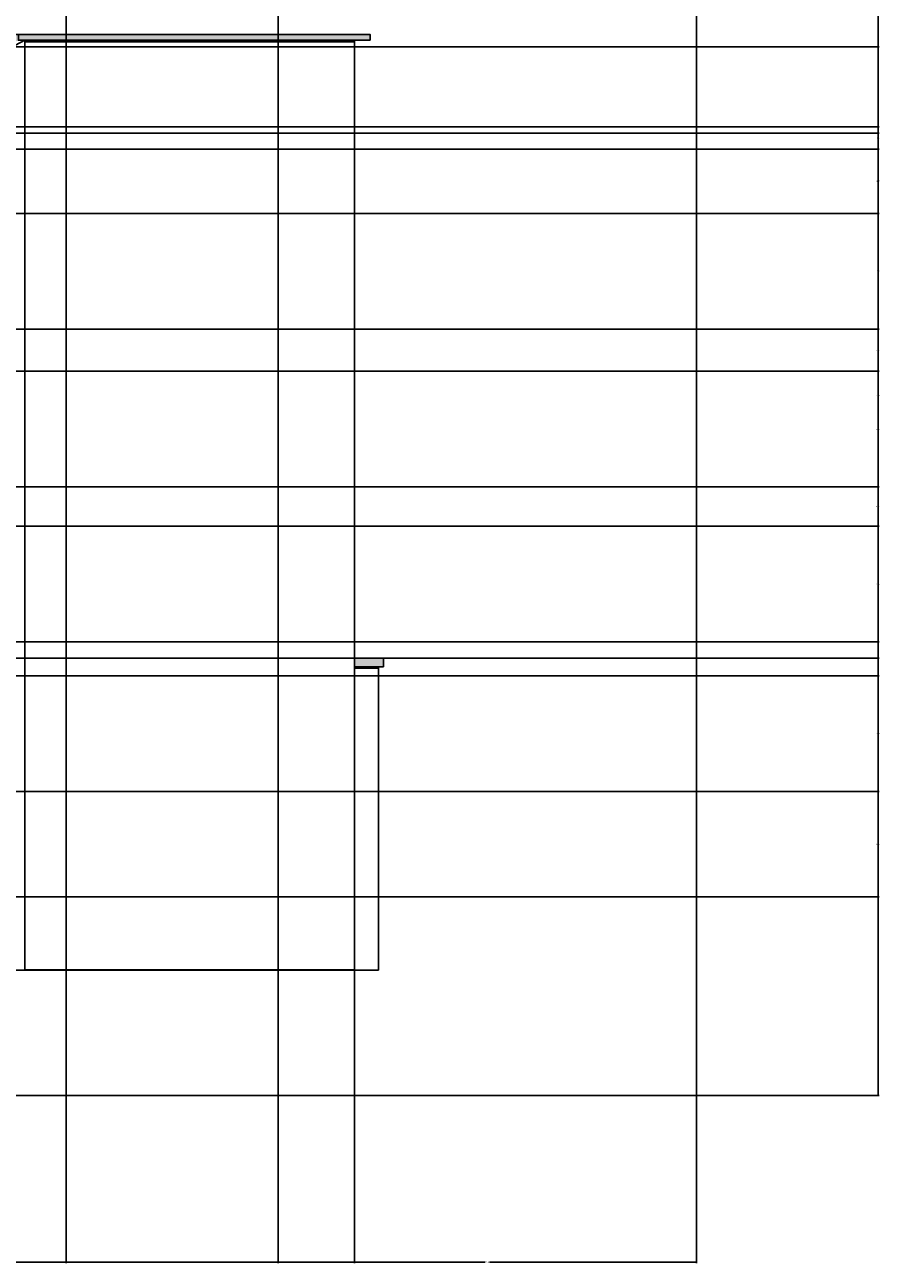
# Model space of a CAD drawing. Units: millimetres. Extents: x 171 to 1599, y 973 to 1509.
# Tile 6 of 7: x 1445 to 1599, y 973 to 1196. Entities that reach past the tile are written whole.
import ezdxf

# ---------------------------------------------------------------- set-up
doc = ezdxf.new("R2010")
doc.units = ezdxf.units.MM
for name, color, linetype, lineweight in [('A-ANNO-DIMS', 2, 'Continuous', 18), ('A-ELEV', 7, 'Continuous', 25), ('A-ELEV-FILL', 252, 'Continuous', 13)]:
    doc.layers.add(name, color=color, linetype=linetype, lineweight=lineweight)
doc.styles.get("Standard").update_dxf_attribs({"font": 'arial.ttf'})
doc.dimstyles.get("Standard").update_dxf_attribs({"dimtxt": 0.18, "dimasz": 0.18, "dimexe": 0.18, "dimexo": 0.0625, "dimgap": 0.09, "dimtad": 0, "dimtih": 1, "dimtoh": 1, "dimdec": 1, "dimzin": 0, "dimdsep": 46, "dimlunit": 3, "dimtxsty": 'Standard', "dimcen": 0.09, "dimadec": 0, "dimazin": 0, "dimtfac": 1, "dimtdec": 1, "dimtofl": 0, "dimtmove": 0, "dimatfit": 3, "dimfxl": 1, "dimtolj": 1, "dimtzin": 0, "dimarcsym": 0})

# ---------------------------------------------------------------- blocks, each defined once
blk = doc.blocks.new('*D1')
at = {"layer": 'A-ANNO-DIMS', "color": 0, "lineweight": -2, "transparency": 16777216}
for p, q in [((980.93, 1194.55), (980.93, 1508.31)), ((981.11, 1508.13), (1274.61, 1508.13)), ((1568.85, 1508.13), (1275.36, 1508.13)), ((1569.03, 1215.31), (1569.03, 1508.31))]:
    blk.add_line(p, q, dxfattribs=at)
at = {"layer": 'A-ANNO-DIMS', "color": 0, "transparency": 16777216}
for points in [[(981.11, 1508.16), (981.11, 1508.1), (980.93, 1508.13)], [(1568.85, 1508.16), (1568.85, 1508.1), (1569.03, 1508.13)]]:
    blk.add_solid(points, dxfattribs=at)
at = {"layer": 'Defpoints', "color": 0, "transparency": 16777216}
for p in [(1569.03, 1508.13), (1569.03, 1215.25), (980.93, 1194.49)]:
    blk.add_point(p, dxfattribs=at)
at = {"layer": 'A-ANNO-DIMS', "color": 0, "transparency": 16777216, "insert": (1274.98, 1508.13), "char_height": 0.18, "attachment_point": 5}
blk.add_mtext('\\A1;588.1', dxfattribs=at)
blk = doc.blocks.new('*D2')
at = {"layer": 'A-ANNO-DIMS', "color": 0, "lineweight": -2, "transparency": 16777216}
for p, q in [((1043.70287, 1478.130098), (1599.212656, 1478.130098)), ((1599.032656, 1477.950098), (1599.032656, 1240.959874)), ((1599.032656, 1003.60965), (1599.032656, 1240.599874)), ((1348.449149, 1003.42965), (1599.212656, 1003.42965))]:
    blk.add_line(p, q, dxfattribs=at)
at = {"layer": 'A-ANNO-DIMS', "color": 0, "transparency": 16777216}
for points in [[(1599.002656, 1477.950098), (1599.062656, 1477.950098), (1599.032656, 1478.130098)], [(1599.002656, 1003.60965), (1599.062656, 1003.60965), (1599.032656, 1003.42965)]]:
    blk.add_solid(points, dxfattribs=at)
at = {"layer": 'Defpoints', "color": 0, "transparency": 16777216}
for p in [(1043.64037, 1478.130098), (1599.032656, 1478.130098), (1348.386649, 1003.42965)]:
    blk.add_point(p, dxfattribs=at)
at = {"layer": 'A-ANNO-DIMS', "color": 0, "transparency": 16777216, "insert": (1599.032656, 1240.779874), "char_height": 0.18, "attachment_point": 5}
blk.add_mtext('\\A1;474.7', dxfattribs=at)
blk = doc.blocks.new('*D10')
at = {"layer": 'A-ANNO-DIMS', "color": 0, "lineweight": -2, "transparency": 16777216}
for p, q in [((1441.28, 1082.17), (1441.28, 973.25)), ((1504.77, 1026.01), (1504.77, 973.25)), ((1441.46, 973.43), (1472.63, 973.43)), ((1504.59, 973.43), (1473.42, 973.43))]:
    blk.add_line(p, q, dxfattribs=at)
at = {"layer": 'A-ANNO-DIMS', "color": 0, "transparency": 16777216}
for points in [[(1441.46, 973.46), (1441.46, 973.4), (1441.28, 973.43)], [(1504.59, 973.46), (1504.59, 973.4), (1504.77, 973.43)]]:
    blk.add_solid(points, dxfattribs=at)
at = {"layer": 'Defpoints', "color": 0, "transparency": 16777216}
for p in [(1441.28, 1082.23), (1504.77, 1026.08), (1504.77, 973.43)]:
    blk.add_point(p, dxfattribs=at)
at = {"layer": 'A-ANNO-DIMS', "color": 0, "transparency": 16777216, "insert": (1473.02, 973.43), "char_height": 0.18, "attachment_point": 5}
blk.add_mtext('\\A1;63.49', dxfattribs=at)
blk = doc.blocks.new('*D58')
at = {"layer": 'A-ANNO-DIMS', "color": 0, "lineweight": -2, "transparency": 16777216}
for p, q in [((1452.86, 1194.43), (1452.86, 973.25)), ((1416.22, 1192.2), (1416.22, 973.25)), ((1416.4, 973.43), (1434.08, 973.43)), ((1452.68, 973.43), (1435, 973.43))]:
    blk.add_line(p, q, dxfattribs=at)
at = {"layer": 'A-ANNO-DIMS', "color": 0, "transparency": 16777216}
for points in [[(1416.4, 973.46), (1416.4, 973.4), (1416.22, 973.43)], [(1452.68, 973.46), (1452.68, 973.4), (1452.86, 973.43)]]:
    blk.add_solid(points, dxfattribs=at)
at = {"layer": 'Defpoints', "color": 0, "transparency": 16777216}
for p in [(1452.86, 1194.49), (1416.22, 1192.27), (1452.86, 973.43)]:
    blk.add_point(p, dxfattribs=at)
at = {"layer": 'A-ANNO-DIMS', "color": 0, "transparency": 16777216, "insert": (1434.54, 973.43), "char_height": 0.18, "attachment_point": 5}
blk.add_mtext('\\A1;36.636', dxfattribs=at)
blk = doc.blocks.new('*D59')
at = {"layer": 'A-ANNO-DIMS', "color": 0, "lineweight": -2, "transparency": 16777216}
for p, q in [((1452.86, 1194.43), (1452.86, 973.25)), ((1491.01, 1194.43), (1491.01, 973.25)), ((1453.04, 973.43), (1471.47, 973.43)), ((1490.83, 973.43), (1472.4, 973.43))]:
    blk.add_line(p, q, dxfattribs=at)
at = {"layer": 'A-ANNO-DIMS', "color": 0, "transparency": 16777216}
for points in [[(1453.04, 973.46), (1453.04, 973.4), (1452.86, 973.43)], [(1490.83, 973.46), (1490.83, 973.4), (1491.01, 973.43)]]:
    blk.add_solid(points, dxfattribs=at)
at = {"layer": 'Defpoints', "color": 0, "transparency": 16777216}
for p in [(1452.86, 1194.49), (1491.01, 1194.49), (1491.01, 973.43)]:
    blk.add_point(p, dxfattribs=at)
at = {"layer": 'A-ANNO-DIMS', "color": 0, "transparency": 16777216, "insert": (1471.94, 973.43), "char_height": 0.18, "attachment_point": 5}
blk.add_mtext('\\A1;38.156', dxfattribs=at)
blk = doc.blocks.new('*D60')
at = {"layer": 'A-ANNO-DIMS', "color": 0, "lineweight": -2, "transparency": 16777216}
for p, q in [((1566.36, 1203.74), (1566.36, 973.25)), ((1491.01, 1194.43), (1491.01, 973.25)), ((1491.19, 973.43), (1528.29, 973.43)), ((1566.18, 973.43), (1529.08, 973.43))]:
    blk.add_line(p, q, dxfattribs=at)
at = {"layer": 'A-ANNO-DIMS', "color": 0, "transparency": 16777216}
for points in [[(1491.19, 973.46), (1491.19, 973.4), (1491.01, 973.43)], [(1566.18, 973.46), (1566.18, 973.4), (1566.36, 973.43)]]:
    blk.add_solid(points, dxfattribs=at)
at = {"layer": 'Defpoints', "color": 0, "transparency": 16777216}
for p in [(1566.36, 1203.8), (1491.01, 1194.49), (1566.36, 973.43)]:
    blk.add_point(p, dxfattribs=at)
at = {"layer": 'A-ANNO-DIMS', "color": 0, "transparency": 16777216, "insert": (1528.69, 973.43), "char_height": 0.18, "attachment_point": 5}
blk.add_mtext('\\A1;75.35', dxfattribs=at)
blk = doc.blocks.new('*D62')
at = {"layer": 'A-ANNO-DIMS', "color": 0, "lineweight": -2, "transparency": 16777216}
for p, q in [((1416.28, 1290.48), (1599.21, 1290.48)), ((1599.03, 1290.3), (1599.03, 1241.56)), ((1599.03, 1192.45), (1599.03, 1241.19)), ((1416.28, 1192.27), (1599.21, 1192.27))]:
    blk.add_line(p, q, dxfattribs=at)
at = {"layer": 'A-ANNO-DIMS', "color": 0, "transparency": 16777216}
for points in [[(1599, 1290.3), (1599.06, 1290.3), (1599.03, 1290.48)], [(1599, 1192.45), (1599.06, 1192.45), (1599.03, 1192.27)]]:
    blk.add_solid(points, dxfattribs=at)
at = {"layer": 'Defpoints', "color": 0, "transparency": 16777216}
for p in [(1416.22, 1290.48), (1599.03, 1290.48), (1416.22, 1192.27)]:
    blk.add_point(p, dxfattribs=at)
at = {"layer": 'A-ANNO-DIMS', "color": 0, "transparency": 16777216, "insert": (1599.03, 1241.38), "char_height": 0.18, "attachment_point": 5}
blk.add_mtext('\\A1;98.22', dxfattribs=at)
blk = doc.blocks.new('*D86')
at = {"layer": 'A-ANNO-DIMS', "color": 0, "lineweight": -2, "transparency": 16777216}
for p, q in [((1441.34, 1176.74), (1599.21, 1176.74)), ((1599.03, 1176.56), (1599.03, 1129.67)), ((1599.03, 1082.41), (1599.03, 1129.31)), ((1441.34, 1082.23), (1599.21, 1082.23))]:
    blk.add_line(p, q, dxfattribs=at)
at = {"layer": 'A-ANNO-DIMS', "color": 0, "transparency": 16777216}
for points in [[(1599, 1176.56), (1599.06, 1176.56), (1599.03, 1176.74)], [(1599, 1082.41), (1599.06, 1082.41), (1599.03, 1082.23)]]:
    blk.add_solid(points, dxfattribs=at)
at = {"layer": 'Defpoints', "color": 0, "transparency": 16777216}
for p in [(1441.28, 1176.74), (1599.03, 1176.74), (1441.28, 1082.23)]:
    blk.add_point(p, dxfattribs=at)
at = {"layer": 'A-ANNO-DIMS', "color": 0, "transparency": 16777216, "insert": (1599.03, 1129.49), "char_height": 0.18, "attachment_point": 5}
blk.add_mtext('\\A1;94.51', dxfattribs=at)
blk = doc.blocks.new('*D87')
at = {"layer": 'A-ANNO-DIMS', "color": 0, "lineweight": -2, "transparency": 16777216}
for p, q in [((1281.3, 1058.21), (1599.21, 1058.21)), ((1599.03, 1058.03), (1599.03, 1048.91)), ((1599.03, 1039.43), (1599.03, 1048.55)), ((1294.3, 1039.25), (1599.21, 1039.25))]:
    blk.add_line(p, q, dxfattribs=at)
at = {"layer": 'A-ANNO-DIMS', "color": 0, "transparency": 16777216}
for points in [[(1599, 1058.03), (1599.06, 1058.03), (1599.03, 1058.21)], [(1599, 1039.43), (1599.06, 1039.43), (1599.03, 1039.25)]]:
    blk.add_solid(points, dxfattribs=at)
at = {"layer": 'Defpoints', "color": 0, "transparency": 16777216}
for p in [(1281.24, 1058.21), (1599.03, 1058.21), (1294.24, 1039.25)]:
    blk.add_point(p, dxfattribs=at)
at = {"layer": 'A-ANNO-DIMS', "color": 0, "transparency": 16777216, "insert": (1599.03, 1048.73), "char_height": 0.18, "attachment_point": 5}
blk.add_mtext('\\A1;18.956', dxfattribs=at)
blk = doc.blocks.new('*D88')
at = {"layer": 'A-ANNO-DIMS', "color": 0, "lineweight": -2, "transparency": 16777216}
for p, q in [((1281.3, 1079.04), (1599.21, 1079.04)), ((1599.03, 1078.86), (1599.03, 1068.8)), ((1599.03, 1058.39), (1599.03, 1068.44)), ((1281.3, 1058.21), (1599.21, 1058.21))]:
    blk.add_line(p, q, dxfattribs=at)
at = {"layer": 'A-ANNO-DIMS', "color": 0, "transparency": 16777216}
for points in [[(1599, 1078.86), (1599.06, 1078.86), (1599.03, 1079.04)], [(1599, 1058.39), (1599.06, 1058.39), (1599.03, 1058.21)]]:
    blk.add_solid(points, dxfattribs=at)
at = {"layer": 'Defpoints', "color": 0, "transparency": 16777216}
for p in [(1281.24, 1079.04), (1599.03, 1079.04), (1281.24, 1058.21)]:
    blk.add_point(p, dxfattribs=at)
at = {"layer": 'A-ANNO-DIMS', "color": 0, "transparency": 16777216, "insert": (1599.03, 1068.62), "char_height": 0.18, "attachment_point": 5}
blk.add_mtext('\\A1;20.833', dxfattribs=at)
blk = doc.blocks.new('*D89')
at = {"layer": 'A-ANNO-DIMS', "color": 0, "lineweight": -2, "transparency": 16777216}
for p, q in [((1281.3, 1085.12), (1599.21, 1085.12)), ((1599.03, 1084.94), (1599.03, 1082.26)), ((1599.03, 1079.22), (1599.03, 1081.9)), ((1281.3, 1079.04), (1599.21, 1079.04))]:
    blk.add_line(p, q, dxfattribs=at)
at = {"layer": 'A-ANNO-DIMS', "color": 0, "transparency": 16777216}
for points in [[(1599, 1084.94), (1599.06, 1084.94), (1599.03, 1085.12)], [(1599, 1079.22), (1599.06, 1079.22), (1599.03, 1079.04)]]:
    blk.add_solid(points, dxfattribs=at)
at = {"layer": 'Defpoints', "color": 0, "transparency": 16777216}
for p in [(1281.24, 1085.12), (1599.03, 1085.12), (1281.24, 1079.04)]:
    blk.add_point(p, dxfattribs=at)
at = {"layer": 'A-ANNO-DIMS', "color": 0, "transparency": 16777216, "insert": (1599.03, 1082.08), "char_height": 0.18, "attachment_point": 5}
blk.add_mtext('\\A1;6.079', dxfattribs=at)
blk = doc.blocks.new('*D90')
at = {"layer": 'A-ANNO-DIMS', "color": 0, "lineweight": -2, "transparency": 16777216}
for p, q in [((1281.3, 1105.95), (1599.21, 1105.95)), ((1599.03, 1105.77), (1599.03, 1095.72)), ((1599.03, 1085.3), (1599.03, 1095.35)), ((1281.3, 1085.12), (1599.21, 1085.12))]:
    blk.add_line(p, q, dxfattribs=at)
at = {"layer": 'A-ANNO-DIMS', "color": 0, "transparency": 16777216}
for points in [[(1599, 1105.77), (1599.06, 1105.77), (1599.03, 1105.95)], [(1599, 1085.3), (1599.06, 1085.3), (1599.03, 1085.12)]]:
    blk.add_solid(points, dxfattribs=at)
at = {"layer": 'Defpoints', "color": 0, "transparency": 16777216}
for p in [(1281.24, 1105.95), (1599.03, 1105.95), (1281.24, 1085.12)]:
    blk.add_point(p, dxfattribs=at)
at = {"layer": 'A-ANNO-DIMS', "color": 0, "transparency": 16777216, "insert": (1599.03, 1095.53), "char_height": 0.18, "attachment_point": 5}
blk.add_mtext('\\A1;20.833', dxfattribs=at)
blk = doc.blocks.new('*D91')
at = {"layer": 'A-ANNO-DIMS', "color": 0, "lineweight": -2, "transparency": 16777216}
for p, q in [((1281.3, 1113.05), (1599.21, 1113.05)), ((1599.03, 1112.87), (1599.03, 1109.68)), ((1599.03, 1106.13), (1599.03, 1109.32)), ((1281.3, 1105.95), (1599.21, 1105.95))]:
    blk.add_line(p, q, dxfattribs=at)
at = {"layer": 'A-ANNO-DIMS', "color": 0, "transparency": 16777216}
for points in [[(1599, 1112.87), (1599.06, 1112.87), (1599.03, 1113.05)], [(1599, 1106.13), (1599.06, 1106.13), (1599.03, 1105.95)]]:
    blk.add_solid(points, dxfattribs=at)
at = {"layer": 'Defpoints', "color": 0, "transparency": 16777216}
for p in [(1281.24, 1113.05), (1599.03, 1113.05), (1281.24, 1105.95)]:
    blk.add_point(p, dxfattribs=at)
at = {"layer": 'A-ANNO-DIMS', "color": 0, "transparency": 16777216, "insert": (1599.03, 1109.5), "char_height": 0.18, "attachment_point": 5}
blk.add_mtext('\\A1;7.102', dxfattribs=at)
blk = doc.blocks.new('*D92')
at = {"layer": 'A-ANNO-DIMS', "color": 0, "lineweight": -2, "transparency": 16777216}
for p, q in [((1281.3, 1133.89), (1599.21, 1133.89)), ((1599.03, 1133.71), (1599.03, 1123.65)), ((1599.03, 1113.23), (1599.03, 1123.29)), ((1281.3, 1113.05), (1599.21, 1113.05))]:
    blk.add_line(p, q, dxfattribs=at)
at = {"layer": 'A-ANNO-DIMS', "color": 0, "transparency": 16777216}
for points in [[(1599, 1133.71), (1599.06, 1133.71), (1599.03, 1133.89)], [(1599, 1113.23), (1599.06, 1113.23), (1599.03, 1113.05)]]:
    blk.add_solid(points, dxfattribs=at)
at = {"layer": 'Defpoints', "color": 0, "transparency": 16777216}
for p in [(1281.24, 1133.89), (1599.03, 1133.89), (1281.24, 1113.05)]:
    blk.add_point(p, dxfattribs=at)
at = {"layer": 'A-ANNO-DIMS', "color": 0, "transparency": 16777216, "insert": (1599.03, 1123.47), "char_height": 0.18, "attachment_point": 5}
blk.add_mtext('\\A1;20.833', dxfattribs=at)
blk = doc.blocks.new('*D93')
at = {"layer": 'A-ANNO-DIMS', "color": 0, "lineweight": -2, "transparency": 16777216}
for p, q in [((1281.3, 1141.45), (1599.21, 1141.45)), ((1599.03, 1141.27), (1599.03, 1137.85)), ((1599.03, 1134.07), (1599.03, 1137.49)), ((1281.3, 1133.89), (1599.21, 1133.89))]:
    blk.add_line(p, q, dxfattribs=at)
at = {"layer": 'A-ANNO-DIMS', "color": 0, "transparency": 16777216}
for points in [[(1599, 1141.27), (1599.06, 1141.27), (1599.03, 1141.45)], [(1599, 1134.07), (1599.06, 1134.07), (1599.03, 1133.89)]]:
    blk.add_solid(points, dxfattribs=at)
at = {"layer": 'Defpoints', "color": 0, "transparency": 16777216}
for p in [(1281.24, 1141.45), (1599.03, 1141.45), (1281.24, 1133.89)]:
    blk.add_point(p, dxfattribs=at)
at = {"layer": 'A-ANNO-DIMS', "color": 0, "transparency": 16777216, "insert": (1599.03, 1137.67), "char_height": 0.18, "attachment_point": 5}
blk.add_mtext('\\A1;7.567', dxfattribs=at)
blk = doc.blocks.new('*D94')
at = {"layer": 'A-ANNO-DIMS', "color": 0, "lineweight": -2, "transparency": 16777216}
for p, q in [((1281.3, 1162.29), (1599.21, 1162.29)), ((1599.03, 1162.11), (1599.03, 1152.05)), ((1599.03, 1141.63), (1599.03, 1151.69)), ((1281.3, 1141.45), (1599.21, 1141.45))]:
    blk.add_line(p, q, dxfattribs=at)
at = {"layer": 'A-ANNO-DIMS', "color": 0, "transparency": 16777216}
for points in [[(1599, 1162.11), (1599.06, 1162.11), (1599.03, 1162.29)], [(1599, 1141.63), (1599.06, 1141.63), (1599.03, 1141.45)]]:
    blk.add_solid(points, dxfattribs=at)
at = {"layer": 'Defpoints', "color": 0, "transparency": 16777216}
for p in [(1281.24, 1162.29), (1599.03, 1162.29), (1281.24, 1141.45)]:
    blk.add_point(p, dxfattribs=at)
at = {"layer": 'A-ANNO-DIMS', "color": 0, "transparency": 16777216, "insert": (1599.03, 1151.87), "char_height": 0.18, "attachment_point": 5}
blk.add_mtext('\\A1;20.833', dxfattribs=at)
blk = doc.blocks.new('*D95')
at = {"layer": 'A-ANNO-DIMS', "color": 0, "lineweight": -2, "transparency": 16777216}
for p, q in [((1294.3, 1173.87), (1599.21, 1173.87)), ((1599.03, 1173.69), (1599.03, 1168.26)), ((1599.03, 1162.47), (1599.03, 1167.9)), ((1281.3, 1162.29), (1599.21, 1162.29))]:
    blk.add_line(p, q, dxfattribs=at)
at = {"layer": 'A-ANNO-DIMS', "color": 0, "transparency": 16777216}
for points in [[(1599, 1173.69), (1599.06, 1173.69), (1599.03, 1173.87)], [(1599, 1162.47), (1599.06, 1162.47), (1599.03, 1162.29)]]:
    blk.add_solid(points, dxfattribs=at)
at = {"layer": 'Defpoints', "color": 0, "transparency": 16777216}
for p in [(1294.24, 1173.87), (1599.03, 1173.87), (1281.24, 1162.29)]:
    blk.add_point(p, dxfattribs=at)
at = {"layer": 'A-ANNO-DIMS', "color": 0, "transparency": 16777216, "insert": (1599.03, 1168.08), "char_height": 0.18, "attachment_point": 5}
blk.add_mtext('\\A1;11.587', dxfattribs=at)
blk = doc.blocks.new('*D96')
at = {"layer": 'A-ANNO-DIMS', "color": 0, "lineweight": -2, "transparency": 16777216}
for p, q in [((1298.3, 1177.87), (1599.21, 1177.87)), ((1599.03, 1177.69), (1599.03, 1176.05)), ((1599.03, 1174.05), (1599.03, 1175.69)), ((1294.3, 1173.87), (1599.21, 1173.87))]:
    blk.add_line(p, q, dxfattribs=at)
at = {"layer": 'A-ANNO-DIMS', "color": 0, "transparency": 16777216}
for points in [[(1599, 1177.69), (1599.06, 1177.69), (1599.03, 1177.87)], [(1599, 1174.05), (1599.06, 1174.05), (1599.03, 1173.87)]]:
    blk.add_solid(points, dxfattribs=at)
at = {"layer": 'Defpoints', "color": 0, "transparency": 16777216}
for p in [(1298.24, 1177.87), (1599.03, 1177.87), (1294.24, 1173.87)]:
    blk.add_point(p, dxfattribs=at)
at = {"layer": 'A-ANNO-DIMS', "color": 0, "transparency": 16777216, "insert": (1599.03, 1175.87), "char_height": 0.18, "attachment_point": 5}
blk.add_mtext('\\A1;4.00', dxfattribs=at)

msp = doc.modelspace()

# ---------------------------------------------------------------- hatches: boundary and pattern name
at = {"layer": 'A-ELEV-FILL'}
h = msp.add_hatch(color=256, dxfattribs=at)
h.dxf.hatch_style = 1
h.paths.add_polyline_path([(1507.6024, 1194.488), (1444.2789, 1194.488), (1444.2789, 1193.4707), (1507.6024, 1193.4707)])
h.paths.add_polyline_path([(1444.2789, 1193.4707), (1444.2789, 1194.488), (1440.129, 1192.267), (1440.129, 1191.2497)])
h = msp.add_hatch(color=256, dxfattribs=at)
h.dxf.hatch_style = 1
h.paths.add_polyline_path([(1057.1375, 1082.2327), (1051.6226, 1082.2327), (1051.6226, 1080.6718), (1057.1375, 1080.6718)])
h.paths.add_polyline_path([(1143.7, 1082.2327), (1057.1375, 1082.2327), (1057.1375, 1080.6718), (1143.7, 1080.6718)])
h.paths.add_polyline_path([(1509.9876, 1082.2327), (1504.7689, 1082.2327), (1504.7689, 1080.6718), (1509.0669, 1080.6718), (1509.9876, 1080.6718)])
h.paths.add_polyline_path([(1443.1972, 1082.2327), (1328.4737, 1082.2327), (1328.4737, 1080.6718), (1329.4402, 1080.6718), (1443.1972, 1080.6718)])

# ---------------------------------------------------------------- linework, layer by layer
at = {"layer": 'A-ELEV'}
for p, q in [((1507.6024, 1194.488), (1440.129, 1194.488)), ((1441.2762, 1191.2497), (1445.4261, 1193.4707)), ((1504.7689, 1193.222), (1445.4261, 1193.222)), ((1504.7689, 1193.4707), (1504.7689, 1193.222)), ((1507.6024, 1193.4707), (1507.6024, 1194.488)), ((1504.7689, 1080.3893), (1509.0669, 1080.3893)), ((1340.5107, 1026.0387), (1509.0669, 1026.0387))]:
    msp.add_line(p, q, dxfattribs=at)
for points in [[(1491.0132, 1247.3037), (1491.0132, 1194.488), (1452.8572, 1194.488), (1452.8572, 1269.3331)], [(1509.0669, 1080.6718), (1509.9876, 1080.6718), (1509.9876, 1082.2327), (1504.7689, 1082.2327)], [(1504.7689, 1080.6718), (1509.0669, 1080.6718), (1509.0669, 1026.0387), (1340.5107, 1026.0387)]]:
    msp.add_lwpolyline(points, dxfattribs=at)
for points in [[(1507.6024, 1193.4707), (1444.2789, 1193.4707), (1444.2789, 1194.488), (1507.6024, 1194.488)], [(1504.7689, 1026.0766), (1445.4261, 1026.0766), (1445.4261, 1193.4707), (1504.7689, 1193.4707)]]:
    msp.add_lwpolyline(points, close=True, dxfattribs=at)

# ---------------------------------------------------------------- dimensions: what is measured, and where the dimension line sits
at = {"layer": 'A-ANNO-DIMS'}
for base, p1, p2, override, picture, middle in [((1569.0327, 1508.1301), (980.9303, 1194.488), (1569.0327, 1215.2519), {"dimdec": 1, "dimlfac": 1, "dimrnd": 0, "dimzin": 0, "dimdsep": 46, "dimlunit": 2}, '*D1', (1274.9815, 1508.1301)), ((1566.3585, 973.4297), (1491.0132, 1194.488), (1566.3585, 1203.8031), {"dimdec": 2, "dimlfac": 1, "dimrnd": 0, "dimzin": 0, "dimdsep": 46, "dimlunit": 2}, '*D60', (1528.6858, 973.4297)), ((1452.8572, 973.4297), (1416.2216, 1192.267), (1452.8572, 1194.488), {"dimdec": 3, "dimlfac": 1, "dimrnd": 0, "dimzin": 0, "dimdsep": 46, "dimlunit": 2}, '*D58', (1434.5394, 973.4297)), ((1491.0132, 973.4297), (1452.8572, 1194.488), (1491.0132, 1194.488), {"dimdec": 3, "dimlfac": 1, "dimrnd": 0, "dimzin": 0, "dimdsep": 46, "dimlunit": 2}, '*D59', (1471.9352, 973.4297)), ((1504.7689, 973.4297), (1441.2762, 1082.2327), (1504.7689, 1026.0766), {"dimdec": 2, "dimlfac": 1, "dimrnd": 0, "dimzin": 0, "dimdsep": 46, "dimlunit": 2}, '*D10', (1473.0225, 973.4297))]:
    dim = msp.add_linear_dim(base=base, p1=p1, p2=p2, dimstyle='Standard', override=override, dxfattribs=at)
    dim.commit()
    dim.dimension.update_dxf_attribs({"geometry": picture, "text_midpoint": middle})
for base, p1, p2, override, picture, middle in [((1599.0327, 1478.1301), (1348.3866, 1003.4297), (1043.6404, 1478.1301), {"dimdec": 1, "dimlfac": 1, "dimrnd": 0, "dimzin": 0, "dimdsep": 46, "dimlunit": 2}, '*D2', (1599.0327, 1240.7799)), ((1599.0327, 1290.4846), (1416.2216, 1192.267), (1416.2216, 1290.4846), {"dimdec": 2, "dimlfac": 1, "dimrnd": 0, "dimzin": 0, "dimdsep": 46, "dimlunit": 2}, '*D62', (1599.0327, 1241.3758)), ((1599.0327, 1177.8722), (1294.2363, 1173.8722), (1298.2363, 1177.8722), {"dimdec": 2, "dimlfac": 1, "dimrnd": 0, "dimzin": 0, "dimdsep": 46, "dimlunit": 2}, '*D96', (1599.0327, 1175.8722)), ((1599.0327, 1176.7441), (1441.2762, 1082.2327), (1441.2762, 1176.7441), {"dimdec": 2, "dimlfac": 1, "dimrnd": 0, "dimzin": 0, "dimdsep": 46, "dimlunit": 2}, '*D86', (1599.0327, 1129.4884)), ((1599.0327, 1173.8722), (1281.2416, 1162.2854), (1294.2363, 1173.8722), {"dimdec": 3, "dimlfac": 1, "dimrnd": 0, "dimzin": 0, "dimdsep": 46, "dimlunit": 2}, '*D95', (1599.0327, 1168.0788)), ((1599.0327, 1162.2854), (1281.2416, 1141.4523), (1281.2416, 1162.2854), {"dimdec": 3, "dimlfac": 1, "dimrnd": 0, "dimzin": 0, "dimdsep": 46, "dimlunit": 2}, '*D94', (1599.0327, 1151.8688)), ((1599.0327, 1141.4523), (1281.2416, 1133.885), (1281.2416, 1141.4523), {"dimdec": 3, "dimlfac": 1, "dimrnd": 0, "dimzin": 0, "dimdsep": 46, "dimlunit": 2}, '*D93', (1599.0327, 1137.6687)), ((1599.0327, 1133.885), (1281.2416, 1113.0519), (1281.2416, 1133.885), {"dimdec": 3, "dimlfac": 1, "dimrnd": 0, "dimzin": 0, "dimdsep": 46, "dimlunit": 2}, '*D92', (1599.0327, 1123.4685)), ((1599.0327, 1113.0519), (1281.2416, 1105.9503), (1281.2416, 1113.0519), {"dimdec": 3, "dimlfac": 1, "dimrnd": 0, "dimzin": 0, "dimdsep": 46, "dimlunit": 2}, '*D91', (1599.0327, 1109.5011)), ((1599.0327, 1105.9503), (1281.2416, 1085.1172), (1281.2416, 1105.9503), {"dimdec": 3, "dimlfac": 1, "dimrnd": 0, "dimzin": 0, "dimdsep": 46, "dimlunit": 2}, '*D90', (1599.0327, 1095.5337)), ((1599.0327, 1085.1172), (1281.2416, 1079.0383), (1281.2416, 1085.1172), {"dimdec": 3, "dimlfac": 1, "dimrnd": 0, "dimzin": 0, "dimdsep": 46, "dimlunit": 2}, '*D89', (1599.0327, 1082.0777)), ((1599.0327, 1079.0383), (1281.2416, 1058.2052), (1281.2416, 1079.0383), {"dimdec": 3, "dimlfac": 1, "dimrnd": 0, "dimzin": 0, "dimdsep": 46, "dimlunit": 2}, '*D88', (1599.0327, 1068.6217)), ((1599.0327, 1058.2052), (1294.2363, 1039.2493), (1281.2416, 1058.2052), {"dimdec": 3, "dimlfac": 1, "dimrnd": 0, "dimzin": 0, "dimdsep": 46, "dimlunit": 2}, '*D87', (1599.0327, 1048.7272))]:
    dim = msp.add_linear_dim(base=base, p1=p1, p2=p2, angle=90, dimstyle='Standard', override=override, dxfattribs=at)
    dim.commit()
    dim.dimension.update_dxf_attribs({"geometry": picture, "text_midpoint": middle})

doc.saveas('drawing.dxf')
